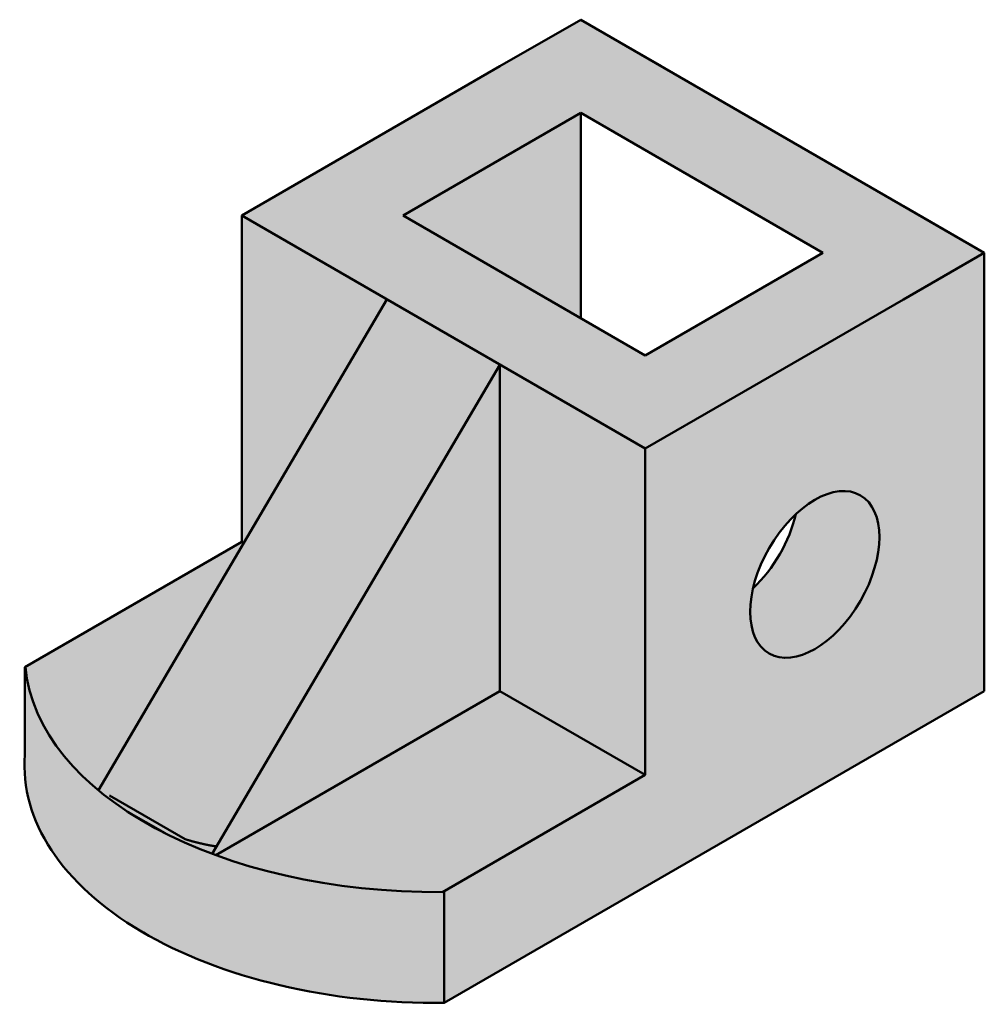
# Model space of a CAD drawing. Units: millimetres. Extents: x 82 to 186, y 61 to 166.
import ezdxf

# ---------------------------------------------------------------- set-up
doc = ezdxf.new("R2010")
doc.units = ezdxf.units.MM
doc.header["$MEASUREMENT"] = 0
doc.layers.add('M-HATC', color=7, linetype='Continuous', lineweight=18)
doc.layers.add('M-OUTL', color=7, linetype='Continuous', lineweight=50)

msp = doc.modelspace()

# ---------------------------------------------------------------- hatches: boundary and pattern name
at = {"layer": 'M-HATC'}
h = msp.add_hatch(color=256, dxfattribs=at)
h.dxf.hatch_style = 1
h.set_gradient(color1=(99, 100, 102), name='INVCYLINDER')
edge = h.paths.add_edge_path(flags=0)
edge.add_ellipse((167.3173071630044, 106.8724986892286), major_axis=(-4.898979485566359, -8.485281374238568), ratio=0.5773502691896244, start_angle=312.5057290122221, end_angle=227.4942709877777)
edge.add_ellipse((158.65705312516, 111.8724986892286), major_axis=(-4.898979485566359, -8.485281374238568), ratio=0.5773502691896244, start_angle=47.49427098777801, end_angle=132.5057290122221, ccw=False)
edge = h.paths.add_edge_path()
edge.add_line((185.5038406424776, 141.3724986892286), (176.8435866046332, 136.3724986892286))
edge.add_line((176.8435866046332, 136.3724986892286), (157.7910277213756, 125.3724986892286))
edge.add_line((157.7910277213756, 125.3724986892286), (149.1307736835312, 120.3724986892286))
edge.add_line((149.1307736835312, 120.3724986892286), (149.1307736835312, 85.37249868922864))
edge.add_line((149.1307736835312, 85.37249868922864), (127.380191469522, 72.81479419293936))
edge.add_ellipse((126.6587430033003, 98.26723030496724), major_axis=(-44.09081537009717, 0), ratio=0.577350269189626, start_angle=402.32299623731546, end_angle=451.6236122594404, ccw=False)
edge.add_ellipse((126.6587430033003, 98.26723030496724), major_axis=(-44.09081537009717, 0), ratio=0.577350269189626, start_angle=401.69533367865506, end_angle=402.32299623731546, ccw=False)
edge.add_ellipse((126.6587430033003, 98.26723030496724), major_axis=(-44.09081537009717, 0), ratio=0.577350269189626, start_angle=393.4128070903051, end_angle=401.69533367865506, ccw=False)
edge.add_ellipse((126.6587430033003, 98.26723030496724), major_axis=(-44.09081537009717, 0), ratio=0.577350269189626, start_angle=386.8065907750446, end_angle=393.4128070903051, ccw=False)
edge.add_ellipse((126.6587430033003, 98.26723030496724), major_axis=(-44.09081537009717, 0), ratio=0.577350269189626, start_angle=381.8676338140084, end_angle=386.8065907750446, ccw=False)
edge.add_ellipse((126.6587430033003, 98.26723030496724), major_axis=(-44.09081537009717, 0), ratio=0.577350269189626, start_angle=361.6806317781145, end_angle=381.8676338140084, ccw=False)
edge.add_line((82.62475377750052, 96.97523019375117), (82.56913927297722, 96.94312114459382))
edge.add_line((82.56913927297722, 96.94312114459382), (82.56913927297722, 87.5374045716534))
edge.add_ellipse((126.6137476815596, 86.37229082404068), major_axis=(-44.09081537009717, 0), ratio=0.577350269189626, start_angle=358.4847058883952, end_angle=389.7612071225407)
edge.add_line((95.28679690331504, 68.45933317752642), (95.5875949239661, 68.28566735933175))
edge.add_ellipse((126.6137476815596, 86.37229082404068), major_axis=(-44.09081537009717, 0), ratio=0.577350269189626, start_angle=390.2399476116062, end_angle=452.144069765684)
edge.add_line((127.5665551184747, 60.92239129582932), (185.5038406424776, 94.37249868922864))
edge.add_line((185.5038406424776, 94.37249868922864), (185.5038406424776, 141.3724986892286))
edge = h.paths.add_edge_path(flags=16)
edge.add_ellipse((167.3173071630044, 106.8724986892286), major_axis=(-4.898979485566359, -8.485281374238568), ratio=0.5773502691896244, start_angle=227.4942709877778, end_angle=312.50572901222216, ccw=False)
edge.add_ellipse((167.3173071630044, 106.8724986892286), major_axis=(-4.898979485566359, -8.485281374238568), ratio=0.5773502691896244, start_angle=312.50572901222216, end_angle=587.4942709877777, ccw=False)
edge = h.paths.add_edge_path(flags=17)
edge.add_line((149.1307736835312, 85.37249868922864), (133.5423164154113, 94.37249868922862))
edge.add_line((133.5423164154113, 94.37249868922862), (103.050456066965, 76.76801490896067))
edge.add_ellipse((126.6587430033003, 98.26723030496724), major_axis=(-44.09081537009717, 0), ratio=0.577350269189626, start_angle=402.3229962373155, end_angle=451.6236122594404)
edge.add_line((127.380191469522, 72.81479419293936), (149.1307736835312, 85.37249868922864))
edge = h.paths.add_edge_path(flags=17)
edge.add_line((133.5423164154113, 129.3724986892286), (121.4179607624291, 136.3724986892286))
edge.add_line((121.4179607624291, 136.3724986892286), (90.45573536072811, 83.73746502088164))
edge.add_ellipse((126.6587430033003, 98.26723030496724), major_axis=(-44.09081537009717, 0), ratio=0.577350269189626, start_angle=381.8676338140083, end_angle=386.8065907750446)
edge.add_line((93.47984974276056, 81.50257460708394), (97.62150756316714, 79.11138734958098))
edge.add_ellipse((126.6587430033003, 98.26723030496724), major_axis=(-44.09081537009717, 0), ratio=0.577350269189626, start_angle=393.412807090305, end_angle=401.695333678655)
edge.add_line((102.6789428593095, 76.90551076545562), (133.5423164154113, 129.3724986892286))
edge = h.paths.add_edge_path(flags=17)
edge.add_line((133.5423164154113, 129.3724986892286), (102.6789428593095, 76.9055107654556))
edge.add_ellipse((126.6587430033003, 98.26723030496724), major_axis=(-44.09081537009717, 0), ratio=0.577350269189626, start_angle=401.695333678655, end_angle=402.3229962373155)
edge.add_line((103.050456066965, 76.76801490896067), (133.5423164154113, 94.37249868922862))
edge.add_line((133.5423164154113, 94.37249868922862), (133.5423164154113, 129.3724986892286))
h.paths.add_polyline_path([(149.1307736835312, 120.3724986892286), (133.5423164154113, 129.3724986892286), (133.5423164154113, 94.37249868922862), (149.1307736835312, 85.37249868922864)], flags=17)
edge = h.paths.add_edge_path(flags=17)
edge.add_line((106.04905923048, 110.2457381258483), (105.8295034943093, 110.3724986892286))
edge.add_line((105.8295034943093, 110.3724986892286), (82.62475377750053, 96.97523019375117))
edge.add_ellipse((126.6587430033003, 98.26723030496724), major_axis=(-44.09081537009717, 0), ratio=0.577350269189626, start_angle=361.6806317781145, end_angle=381.8676338140083)
edge.add_line((90.45573536072811, 83.73746502088164), (106.04905923048, 110.2457381258483))
h.paths.add_polyline_path([(121.4179607624291, 136.3724986892286), (105.8295034943093, 145.3724986892286), (105.8295034943093, 110.3724986892286), (106.04905923048, 110.2457381258483)])
h.paths.add_polyline_path([(176.8435866046333, 146.3724986892286), (142.2025704532557, 166.3724986892286), (133.5423164154113, 161.3724986892286), (114.4897575321536, 150.3724986892286), (105.8295034943093, 145.3724986892286), (121.4179607624291, 136.3724986892286), (133.5423164154113, 129.3724986892286), (149.1307736835312, 120.3724986892286), (157.7910277213756, 125.3724986892286), (176.8435866046332, 136.3724986892286), (185.5038406424776, 141.3724986892286)])
h.paths.add_polyline_path([(123.1500115699979, 145.3724986892286), (142.2025704532557, 156.3724986892286), (168.1833325667888, 141.3724986892286), (149.1307736835312, 130.3724986892286)], flags=16)
h.paths.add_polyline_path([(142.2025704532557, 156.3724986892286), (123.1500115699979, 145.3724986892286), (142.2025704532557, 134.3724986892285)], flags=0)
h = msp.add_hatch(color=256, dxfattribs=at)
h.dxf.hatch_style = 1
h.set_gradient(color1=(99, 100, 102), name='INVCYLINDER')
h.paths.add_polyline_path([(142.2025704532557, 156.3724986892286), (123.150011569998, 145.3724986892286), (142.2025704532557, 134.3724986892286)])
edge = h.paths.add_edge_path()
edge.add_ellipse((167.3173071630044, 106.8724986892286), major_axis=(-4.898979485566359, -8.485281374238568), ratio=0.5773502691896244, start_angle=312.5057290122221, end_angle=227.4942709877777)
edge.add_ellipse((158.65705312516, 111.8724986892286), major_axis=(-4.898979485566359, -8.485281374238568), ratio=0.5773502691896244, start_angle=47.49427098777801, end_angle=132.5057290122221, ccw=False)

# ---------------------------------------------------------------- linework, layer by layer
at = {"layer": 'M-OUTL'}
for p, q in [((133.5423164154113, 161.3724986892286), (142.2025704532557, 166.3724986892286)), ((142.2025704532557, 166.3724986892286), (185.5038406424776, 141.3724986892286)), ((142.2025704532557, 166.3724986892286), (150.8628244911001, 161.3724986892286)), ((114.4897575321536, 150.3724986892286), (133.5423164154113, 161.3724986892286)), ((142.2025704532557, 156.3724986892286), (123.150011569998, 145.3724986892286)), ((142.2025704532557, 156.3724986892286), (168.1833325667888, 141.3724986892286)), ((142.2025704532557, 156.3724986892286), (142.2025704532557, 134.3724986892286)), ((105.8295034943093, 145.3724986892286), (114.4897575321536, 150.3724986892286)), ((185.5038406424776, 141.3724986892286), (176.8435866046333, 146.3724986892286)), ((149.1307736835312, 120.3724986892286), (105.8295034943093, 145.3724986892286)), ((105.8295034943093, 145.3724986892286), (105.8295034943093, 110.3724986892286)), ((123.1500115699981, 145.3724986892286), (149.1307736835312, 130.3724986892286)), ((168.1833325667889, 141.3724986892286), (149.1307736835312, 130.3724986892286)), ((185.5038406424776, 141.3724986892286), (176.8435866046332, 136.3724986892286)), ((185.5038406424776, 94.37249868922865), (185.5038406424776, 141.3724986892286)), ((121.4179607624291, 136.3724986892286), (90.45573536072811, 83.73746502088164)), ((176.8435866046332, 136.3724986892286), (157.7910277213756, 125.3724986892286)), ((133.5423164154113, 129.3724986892286), (102.6789428593095, 76.90551076545562)), ((133.5423164154113, 129.3724986892286), (133.5423164154113, 94.37249868922862)), ((157.7910277213756, 125.3724986892286), (149.1307736835312, 120.3724986892286)), ((149.1307736835312, 120.3724986892286), (149.1307736835312, 85.3724986892286)), ((82.56913927297722, 96.94312114459382), (105.8295034943093, 110.3724986892286)), ((105.8295034943093, 110.3724986892286), (106.04905923048, 110.2457381258483)), ((106.04905923048, 110.2457381258483), (105.8295034943093, 110.3724986892286)), ((82.56913927297722, 87.53740457165382), (82.56913927297722, 96.94312114459382)), ((133.5423164154113, 94.37249868922862), (103.050456066965, 76.76801490896067)), ((127.5665551184747, 60.92239129582933), (185.5038406424776, 94.37249868922864)), ((133.5423164154113, 94.37249868922862), (149.1307736835312, 85.3724986892286)), ((127.380191469522, 72.81479419293936), (149.1307736835312, 85.3724986892286)), ((99.77666634106404, 78.47451482914319), (91.62972316455252, 83.17815466517472)), ((97.62150756316726, 79.11138734958082), (93.47984974276073, 81.50257460708386)), ((127.5656150494387, 72.92204218813362), (127.5656150494387, 60.9220421881336)), ((95.58759492396477, 68.28566735933259), (95.28679690331779, 68.45933317752484))]:
    msp.add_line(p, q, dxfattribs=at)
msp.add_lwpolyline([(99.77666634106404, 78.47451482914319), (99.81066565123889, 78.46410483889399), (99.84466496141371, 78.45369484864479), (99.87866427158856, 78.4432848583956), (99.91266358176335, 78.4328748681464), (99.94666289193825, 78.42246487789718), (99.98066220211304, 78.41205488764798), (100.0146860023186, 78.40169550012499), (100.0488567427086, 78.39163972895912), (100.0830274830986, 78.38158395779323), (100.1171982234887, 78.37152818662736), (100.1513689638787, 78.36147241546146), (100.1855397042687, 78.3514166442956), (100.2197104446587, 78.34136087312972), (100.2539297337108, 78.3314064343685), (100.2882703944182, 78.32170532661891), (100.3226110551257, 78.31200421886932), (100.3569517158331, 78.30230311111974), (100.3912923765406, 78.29260200337015), (100.425633037248, 78.28290089562057), (100.4599736979554, 78.27319978787098), (100.4943865313392, 78.26365086244044), (100.528895594958, 78.25430484676863), (100.5634046585769, 78.24495883109682), (100.5979137221957, 78.23561281542504), (100.6324227858145, 78.22626679975326), (100.6669318494334, 78.21692078408147), (100.7014409130522, 78.20757476840966), (100.7360453355649, 78.1984318984801), (100.7707212772479, 78.18944138785719), (100.805397218931, 78.18045087723428), (100.840073160614, 78.17146036661138), (100.8747491022971, 78.16246985598848), (100.9094250439801, 78.15347934536558), (100.9441009856631, 78.14448883474267), (100.9788950315199, 78.13575254005644), (101.0137363190461, 78.12711793174488), (101.0485776065723, 78.1184833234333), (101.0834188940985, 78.10984871512173), (101.1182601816247, 78.10121410681016), (101.1531014691509, 78.0925794984986), (101.1879427566772, 78.08394489018701), (101.2229244496171, 78.07561566803052), (101.2579295434594, 78.0673373435665), (101.2929346373016, 78.05905901910252), (101.3279397311439, 78.05078069463852), (101.3629448249861, 78.04250237017453), (101.3979499188284, 78.03422404571053), (101.4329550126706, 78.02594572124654), (101.4681223660637, 78.01802404642329), (101.5032897194568, 78.01010237160006), (101.5384570728498, 78.0021806967768), (101.5736244262429, 77.99425902195355), (101.608791779636, 77.98633734713033), (101.6439591330291, 77.97841567230708), (101.6791494443672, 77.97054499743737), (101.7144775033762, 77.96298032228881), (101.7498055623851, 77.95541564714027), (101.785133621394, 77.94785097199171), (101.8204616804029, 77.94028629684317), (101.8557897394118, 77.93272162169463), (101.8911177984207, 77.92515694654607), (101.9264913273096, 77.91769436680721), (101.9619785308983, 77.91048702559262), (101.997465734487, 77.90327968437802), (102.0329529380757, 77.89607234316341), (102.0684401416644, 77.88886500194882), (102.1039273452532, 77.8816576607342), (102.1394145488419, 77.8744503195196), (102.1749692852213, 77.8673962579066), (102.2106140653217, 77.86054656909573), (102.2462588454221, 77.85369688028487), (102.2819036255225, 77.84684719147398), (102.3175484056229, 77.83999750266312), (102.3531931857233, 77.83314781385226), (102.3888379658236, 77.8262981250414), (102.4245718896273, 77.8196529819848), (102.4603726712084, 77.81316124824392), (102.4961734527895, 77.80666951450304), (102.5319742343706, 77.80017778076216), (102.5677750159517, 77.79368604702127), (102.6035757975328, 77.78719431328038), (102.6393765791139, 77.78070257953951), (102.6752876603782, 77.77446673288384), (102.7112428615159, 77.76833324106227), (102.7471980626535, 77.76219974924072), (102.7831532637911, 77.75606625741914), (102.8191084649288, 77.74993276559759), (102.8550636660664, 77.743799273776), (102.891018867204, 77.73766578195446), (102.927105066178, 77.73183958693781), (102.9632130981247, 77.72606460805532), (102.9993211300714, 77.72028962917283), (103.0354291620181, 77.71451465029034), (103.0715371939648, 77.70873967140784), (103.1076452259115, 77.70296469252536), (103.1437532578582, 77.69718971364286)], dxfattribs=at)
msp.add_ellipse((167.3173071630044, 106.8724986892286), major_axis=(-4.898979485566359, -8.485281374238568), ratio=0.5773502691896244, dxfattribs=at)
for centre, major_axis, ratio, start_param, end_param in [((158.65705312516, 111.8724986892286), (-4.898979485566359, -8.485281374238568), 0.5773502691896244, 1.084101371720131, 2.057491281869667), ((158.65705312516, 111.8724986892286), (-4.898979485566359, -8.485281374238568), 0.5773502691896244, 1.084101371720124, 2.05749128186967), ((126.6137476815596, 86.37229082404068), (-44.09081537009717, 0), 0.577350269189626, 11.78055356353424, 11.78139133839026), ((126.6587430033003, 98.26723030496724), (-44.09081537009717, 0), 0.577350269189626, 6.333961681088807, 7.870345147725878), ((126.6137476815596, 86.37229082404068), (-44.09081537009717, 0), 0.577350269189626, 6.237399320909301, 7.875593427818511)]:
    msp.add_ellipse(centre, major_axis=major_axis, ratio=ratio, start_param=start_param, end_param=end_param, dxfattribs=at)

doc.saveas('drawing.dxf')
